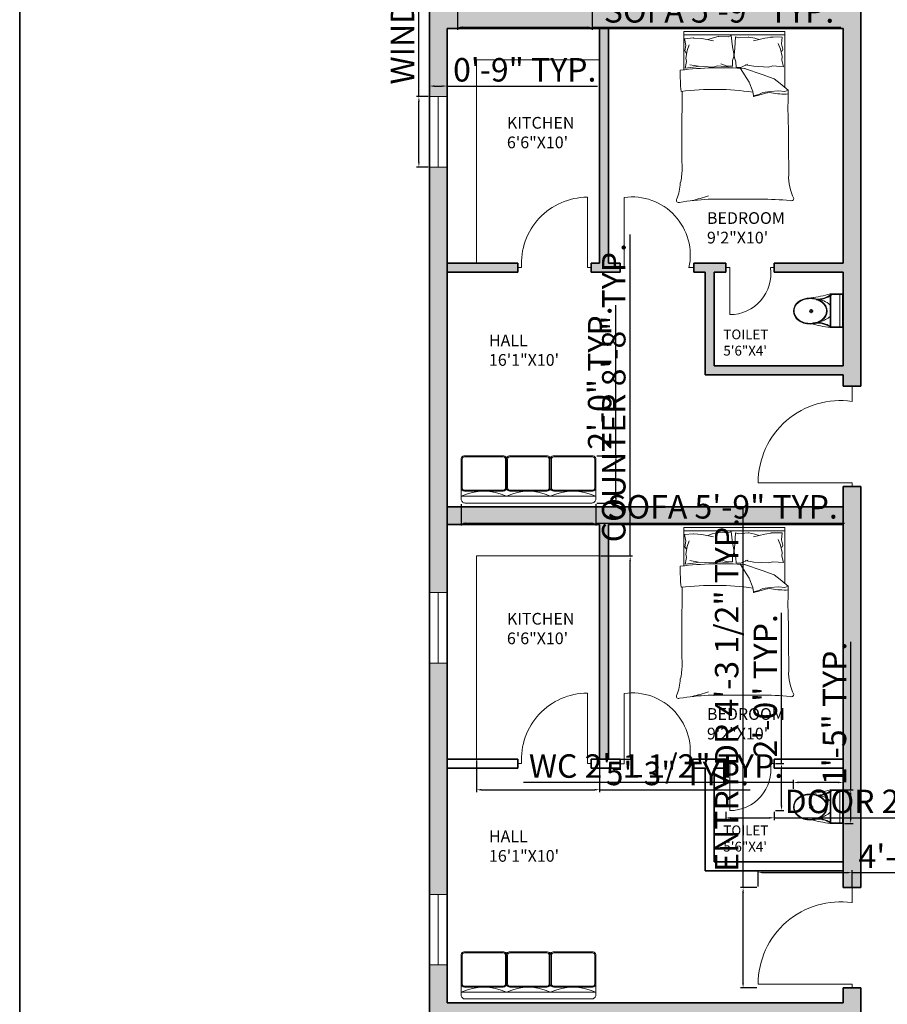
# Model space of a CAD drawing. Units: inches. Extents: x 1266 to 2869, y -408 to 3241.
# Tile 2 of 11: x 1266 to 1710, y 1264 to 1767. Entities that reach past the tile are written whole.
import ezdxf

# ---------------------------------------------------------------- set-up
doc = ezdxf.new("R2010")
doc.units = ezdxf.units.IN
for name, color, linetype, lineweight in [('A-ANNO-DIMS', 2, 'Continuous', 18), ('A-ANNO-TTLB', 7, 'Continuous', 35), ('A-AREA-IDEN', 7, 'Continuous', 18), ('A-DOOR', 4, 'Continuous', 18), ('A-FLOR-CASE', 9, 'Continuous', 18), ('A-FLOR-FIXT', 9, 'Continuous', 18), ('A-FURN', 8, 'Continuous', 18), ('A-GLAZ', 4, 'Continuous', 18), ('A-WALL', 7, 'Continuous', 35), ('A-WALL-PATT', 251, 'Continuous', 13)]:
    doc.layers.add(name, color=color, linetype=linetype, lineweight=lineweight)
doc.styles.get("Standard").update_dxf_attribs({"font": 'arial.ttf'})
doc.dimstyles.new('ISO-25', dxfattribs={"dimtxt": 12, "dimasz": 2.5, "dimexe": 1.25, "dimexo": 0.625, "dimtad": 1, "dimdec": 0, "dimlunit": 3, "dimtxsty": 'Standard', "dimcen": 2.5, "dimadec": 0, "dimazin": 0, "dimtfac": 1, "dimtdec": 0, "dimtmove": 0, "dimatfit": 3, "dimfxl": 1, "dimarcsym": 0})

# ---------------------------------------------------------------- blocks, each defined once
blk = doc.blocks.new('A$C31115884')
for p, q in [((283, 498), (223, 498)), ((258, 466), (258, 523)), ((0, 200), (0, 0)), ((520, 200), (0, 200)), ((10, 190), (10, 10)), ((510, 190), (10, 190)), ((510, 10), (510, 190)), ((520, 0), (520, 200)), ((510, 54), (0, 54)), ((10, 10), (510, 10)), ((0, 0), (520, 0))]:
    blk.add_line(p, q)
blk.add_circle((256, 496), 23.6)
for centre, radius, start, end in [((2778, -205), 2807, 165.4549, 171.7133), ((-295, 403), 365, 324.2091, 9.3499), ((-295, 403), 375, 324.2091, 9.3499), ((806, 403), 365, 170.6501, 215.7909), ((3237, 905), 2807, 188.2867, 194.5451), ((384, 406), 293, 190.2774, 224.1564), ((139, 406), 293, 315.8436, 2.6563), ((806, 403), 375, 179.2036, 215.7909)]:
    blk.add_arc(centre, radius, start, end)
blk.add_ellipse((256, 510), major_axis=(0, -261), ratio=0.772727)
blk.add_open_spline([(256, 259), (263, 259), (270, 260), (288, 262), (299, 265), (320, 273), (330, 278), (350, 291), (360, 299), (378, 316), (386, 326), (402, 347), (409, 358), (421, 383), (427, 395), (436, 422), (440, 436), (445, 465), (447, 480), (448, 509), (448, 524), (445, 553), (443, 568), (436, 596), (432, 610), (422, 636), (416, 649), (402, 672), (395, 683), (379, 703), (370, 712), (351, 728), (341, 735), (321, 746), (310, 751), (289, 757), (278, 759), (256, 761), (245, 761), (223, 757), (212, 754), (191, 746), (181, 741), (161, 728), (151, 720), (133, 703), (125, 693), (110, 672), (103, 660), (90, 636), (85, 623), (76, 596), (72, 582), (67, 553), (66, 538), (64, 509), (65, 494), (68, 465), (70, 450), (77, 422), (81, 408), (91, 382), (97, 370), (111, 346), (118, 335), (135, 316), (144, 307), (162, 291), (172, 284), (193, 273), (203, 269), (225, 262), (236, 260), (250, 259), (253, 259), (256, 259)], degree=3, knots=[0, 0, 0, 0, 0.110105, 0.110105, 0.285049, 0.285049, 0.459994, 0.459994, 0.634938, 0.634938, 0.809882, 0.809882, 0.984827, 0.984827, 1.159771, 1.159771, 1.334715, 1.334715, 1.50966, 1.50966, 1.684604, 1.684604, 1.859549, 1.859549, 2.034493, 2.034493, 2.209437, 2.209437, 2.384382, 2.384382, 2.559326, 2.559326, 2.73427, 2.73427, 2.909215, 2.909215, 3.084159, 3.084159, 3.259103, 3.259103, 3.434048, 3.434048, 3.608992, 3.608992, 3.783936, 3.783936, 3.958881, 3.958881, 4.133825, 4.133825, 4.30877, 4.30877, 4.483714, 4.483714, 4.658658, 4.658658, 4.833603, 4.833603, 5.008547, 5.008547, 5.183491, 5.183491, 5.358436, 5.358436, 5.53338, 5.53338, 5.708324, 5.708324, 5.883269, 5.883269, 6.058213, 6.058213, 6.233158, 6.233158, 6.283185, 6.283185, 6.283185, 6.283185])
blk = doc.blocks.new('BED-DOUBLE')
for p, q in [((3.76, 67.77), (3.76, 87.35)), ((3.76, 87.35), (55.42, 87.35)), ((3.76, 85.69), (55.42, 85.69)), ((55.42, 87.35), (55.42, 58.59)), ((4.21, 83.74), (8.84, 84.1)), ((4.21, 83.77), (4.84, 80.33)), ((5.46, 77.67), (6.55, 80.64)), ((8.84, 84.1), (8.96, 84.08)), ((8.96, 84.08), (13.09, 83.77)), ((13.09, 83.77), (19.03, 82.67)), ((16.06, 83.3), (18.25, 84.08)), ((18.25, 84.08), (21.37, 84.86)), ((21.37, 84.86), (21.72, 84.86)), ((21.72, 84.86), (26.53, 84.7)), ((26.53, 84.7), (28.09, 85.33)), ((28.09, 85.33), (28.71, 79.55)), ((30.24, 84.66), (29.98, 78.85)), ((31.84, 84.13), (30.24, 84.66)), ((36.63, 84.59), (31.84, 84.13)), ((36.98, 84.61), (36.63, 84.59)), ((40.14, 84.02), (36.98, 84.61)), ((45.31, 84.03), (39.45, 82.57)), ((42.38, 83.38), (40.14, 84.02)), ((49.42, 84.6), (45.31, 84.03)), ((54.17, 84.59), (48.33, 84.69)), ((48.33, 84.69), (49.42, 84.6)), ((53.3, 78.43), (52.03, 81.32)), ((54.17, 84.59), (53.76, 81.12)), ((53.76, 81.12), (54.41, 78.34)), ((4.84, 80.33), (4.37, 77.51)), ((4.37, 77.51), (4.99, 76.42)), ((4.84, 73.76), (5.46, 77.67)), ((28.71, 79.55), (29.34, 76.11)), ((29.34, 76.11), (29.34, 74.7)), ((29.98, 78.85), (29.57, 75.38)), ((54.17, 74.56), (53.3, 78.43)), ((54.41, 78.34), (53.85, 77.21)), ((4.52, 68.61), (5.15, 72.04)), ((5.15, 72.04), (4.84, 73.76)), ((26.06, 69.77), (22.66, 70.95)), ((29.34, 74.7), (28.71, 72.67)), ((28.71, 72.67), (28.71, 69.77)), ((29.57, 75.38), (29.66, 73.97)), ((29.66, 73.97), (30.41, 71.98)), ((30.41, 71.98), (30.59, 69.09)), ((33.24, 69.26), (36.56, 70.64)), ((53.97, 72.83), (54.17, 74.56)), ((54.81, 69.44), (53.97, 72.83)), ((10.03, 69.39), (4.52, 68.61)), ((6.9, 70.46), (11.26, 69.74)), ((11.26, 69.74), (10.03, 69.39)), ((11.26, 69.74), (18.84, 69.27)), ((18.84, 69.27), (20.95, 69.87)), ((20.95, 69.87), (26.5, 69.44)), ((28.71, 69.77), (26.06, 69.77)), ((30.59, 69.09), (33.24, 69.26)), ((32.71, 68.56), (37.24, 61.54)), ((43.94, 65.39), (34.92, 68.56)), ((35.2, 70.46), (39.56, 69.74)), ((39.56, 69.74), (47.14, 69.27)), ((47.14, 69.27), (49.26, 69.87)), ((49.26, 69.87), (54.81, 69.44)), ((37.24, 61.54), (39.08, 56.69)), ((49.96, 63.21), (43.94, 65.39)), ((53.15, 60.87), (49.96, 63.21)), ((57.15, 57.36), (53.15, 60.87)), ((39.08, 56.69), (39.42, 54.51)), ((42.1, 55.18), (44.27, 56.19)), ((44.27, 56.19), (47.96, 56.69)), ((47.96, 56.69), (52.14, 57.02)), ((52.14, 57.02), (55.49, 56.69)), ((55.49, 56.69), (57.15, 57.36)), ((57.24, 55.47), (57.15, 57.36, 4.18)), ((39.42, 54.51), (42.1, 55.18)), ((16.28, 1.69), (42.89, 1.69))]:
    blk.add_line(p, q)
for centre, radius, start, end in [((92.06, 65.63), 90.06, 178.7218, 185.604), ((23.09, -109.45), 178.34, 86.0865, 96.7821), ((19.19, -81.63), 139.47, 81.7845, 96.9006), ((-180.86, 53.65), 183.89, 358.4762, 1.0082), ((33.68, 85.75), 32.06, 280.6617, 289.8806), ((47.29, 49.44), 6.73, 78.6608, 113.7384), ((55.49, 94.55), 39.11, 259.8763, 272.5657), ((197.03, 48.09), 139.99, 176.9791, 183.8365), ((39.6, 54.45), 0.199, 160.2464, 271.1377), ((524.11, 32.64), 521.39, 178.2277, 181.7185), ((-4874.07, 14.03), 4931.49, 0.00217, 0.28689), ((-29.08, 17.61), 32.04, 346.0648, 358.9113), ((82.33, 13.12), 24.93, 177.4714, 206.4681), ((-23.41, 11.38), 25.47, 337.9751, 356.652), ((1.18, 1.17), 1.18, 146.1736, 293.4781), ((23.16, -129.76), 131.62, 92.9958, 99.4091), ((-18.62, 112.98), 115.08, 283.3832, 287.7053), ((44.49, -142.13), 143.82, 84.4998, 90.6351), ((58.82, 2.09), 1.19, 242.6588, 356.02)]:
    blk.add_arc(centre, radius, start, end)
blk = doc.blocks.new('SOFA-3-SEAT-3')
for points in [[(0, 22.36), (0, 7.74, 0.414214), (1.72, 6.02), (21.5, 6.02, 0.414214), (23.22, 7.74), (23.22, 22.36, 0.414214), (21.5, 24.08), (1.72, 24.08, 0.414214)], [(0.52, 22.36), (0.52, 7.74, 0.414214), (1.72, 6.54), (21.5, 6.54, 0.414214), (22.7, 7.74), (22.7, 22.36, 0.414214), (21.5, 23.56), (1.72, 23.56, 0.414214)], [(45.57, 22.36), (45.57, 7.74, -0.414214), (43.85, 6.02), (24.94, 6.02, -0.414214), (23.22, 7.74), (23.22, 22.36, -0.414214), (24.94, 24.08), (43.85, 24.08, -0.414214)], [(45.06, 22.36), (45.06, 7.74, -0.414214), (43.85, 6.54), (24.94, 6.54, -0.414214), (23.73, 7.74), (23.73, 22.36, -0.414214), (24.94, 23.56), (43.85, 23.56, -0.414214)], [(45.57, 22.36), (45.57, 7.74, 0.414214), (47.29, 6.02), (67.07, 6.02, 0.414214), (68.79, 7.74), (68.79, 22.36, 0.414214), (67.07, 24.08), (47.29, 24.08, 0.414214)], [(46.09, 22.36), (46.09, 7.74, 0.414214), (47.29, 6.54), (67.07, 6.54, 0.414214), (68.28, 7.74), (68.28, 22.36, 0.414214), (67.07, 23.56), (47.29, 23.56, 0.414214)]]:
    blk.add_lwpolyline(points, format="xyb", close=True)
at = {"ltscale": 0.03}
blk.add_lwpolyline([(21.82, 24.08), (1.38, 24.08, 0.414214), (0, 22.7), (0, 2.06, 0.414214), (2.06, 0), (66.73, 0, 0.414214), (68.79, 2.06), (68.79, 22.7, 0.414214), (67.42, 24.08), (46.97, 24.08, 0.414214), (45.59, 22.7, -1), (45.56, 22.7, 0.414214), (44.18, 24.08), (24.61, 24.08, 0.414214), (23.23, 22.7, -1), (23.2, 22.7, 0.414214)], format="xyb", close=True, dxfattribs=at)
blk.add_lwpolyline([(0, 3.44), (68.79, 3.44)])
for centre, radius, start, end in [((11.61, -21.35), 27.38, 64.9106, 115.0894), ((34.4, -19.35), 25.38, 63.869, 116.131), ((57.18, -21.07), 27.12, 64.6538, 115.3462)]:
    blk.add_arc(centre, radius, start, end)
blk = doc.blocks.new('DOOR-KITCHEN-L')
for p, q in [((35.61, 0), (35.61, 36)), ((0, 0), (2, 0)), ((37.61, 0), (35.61, 0))]:
    blk.add_line(p, q)
blk.add_arc((35.61, 2.31), 33.69, 90, 183.9263)
blk = doc.blocks.new('DOOR-BEDROOM-L')
for p, q in [((2, 0), (2, 36)), ((0, 0), (2, 0)), ((37.12, 0.11), (35.12, 0.11))]:
    blk.add_line(p, q)
blk.add_arc((5.98, 6.45), 29.82, 347.7222, 97.6759)
blk = doc.blocks.new('DOOR-BATH-L')
for p, q in [((0, 24), (2, 24)), ((2, 24), (2, 0)), ((24.7, 24), (22.7, 24))]:
    blk.add_line(p, q)
blk.add_arc((2, 20.92), 20.92, 270, 8.4511)
blk = doc.blocks.new('DOOR-ENTRY-L')
for p, q in [((48, 51.27), (48, 45.59)), ((48, 45.59), (48, 43.59)), ((12, 2), (0, 2)), ((48, 2), (12, 2)), ((48, 0), (48, 2))]:
    blk.add_line(p, q)
blk.add_arc((42.02, 2), 42.02, 81.8116, 180)
blk = doc.blocks.new('WIN-PLAN-36')
for p, q in [((0, 36), (9, 36)), ((4.5, 36), (4.5, 0)), ((9, 36), (4.5, 36)), ((4.5, 0), (0, 0)), ((0, 0), (9, 0))]:
    blk.add_line(p, q)
blk = doc.blocks.new('COUNTER-KITCHEN-2')
for p, q in [((0, 0), (0, 103.95)), ((0, 103.95), (63, 103.95))]:
    blk.add_line(p, q)
blk = doc.blocks.new('*D31')
at = {"layer": 'A-ANNO-DIMS', "color": 0, "lineweight": -2, "transparency": 16777216}
for p, q in [((1470.29, 1727.52), (1470.29, 1883.12)), ((1475.07, 1727.52), (1469.04, 1727.52)), ((1470.29, 1694.02), (1470.29, 1725.02)), ((1475.07, 1691.52), (1469.04, 1691.52))]:
    blk.add_line(p, q, dxfattribs=at)
at = {"layer": 'A-ANNO-DIMS', "color": 0, "transparency": 16777216}
for points in [[(1469.88, 1725.02), (1470.71, 1725.02), (1470.29, 1727.52)], [(1469.88, 1694.02), (1470.71, 1694.02), (1470.29, 1691.52)]]:
    blk.add_solid(points, dxfattribs=at)
at = {"layer": 'Defpoints', "color": 0, "transparency": 16777216}
for p in [(1470.29, 1727.52), (1475.69, 1727.52), (1475.69, 1691.52)]:
    blk.add_point(p, dxfattribs=at)
at = {"layer": 'A-ANNO-DIMS', "color": 0, "transparency": 16777216, "insert": (1463.45, 1806.57), "char_height": 12, "attachment_point": 5, "rotation": 90}
blk.add_mtext('WINDOW 3\'-0" TYP.', dxfattribs=at)
blk = doc.blocks.new('*D32')
at = {"layer": 'A-ANNO-DIMS', "color": 0, "lineweight": -2, "transparency": 16777216}
for p, q in [((1475.69, 1728.15), (1475.69, 1734.17)), ((1478.19, 1732.92), (1482.19, 1732.92)), ((1484.69, 1728.15), (1484.69, 1734.17)), ((1484.69, 1732.92), (1561.59, 1732.92))]:
    blk.add_line(p, q, dxfattribs=at)
at = {"layer": 'A-ANNO-DIMS', "color": 0, "transparency": 16777216}
for points in [[(1478.19, 1733.34), (1478.19, 1732.51), (1475.69, 1732.92)], [(1482.19, 1733.34), (1482.19, 1732.51), (1484.69, 1732.92)]]:
    blk.add_solid(points, dxfattribs=at)
at = {"layer": 'Defpoints', "color": 0, "transparency": 16777216}
for p in [(1484.69, 1732.92), (1475.69, 1727.52), (1484.69, 1727.52)]:
    blk.add_point(p, dxfattribs=at)
at = {"layer": 'A-ANNO-DIMS', "color": 0, "transparency": 16777216, "insert": (1524.39, 1739.68), "char_height": 12, "attachment_point": 5}
blk.add_mtext('0\'-9" TYP.', dxfattribs=at)
blk = doc.blocks.new('*D33')
at = {"layer": 'A-ANNO-DIMS', "color": 0, "lineweight": -2, "transparency": 16777216}
for p, q in [((1661.71, 1376.98), (1523.78, 1376.98)), ((1661.71, 1373.78), (1661.71, 1378.23)), ((1684.69, 1376.98), (1664.21, 1376.98)), ((1687.19, 1373.78), (1687.19, 1378.23))]:
    blk.add_line(p, q, dxfattribs=at)
at = {"layer": 'A-ANNO-DIMS', "color": 0, "transparency": 16777216}
for points in [[(1664.21, 1377.4), (1664.21, 1376.56), (1661.71, 1376.98)], [(1684.69, 1377.4), (1684.69, 1376.56), (1687.19, 1376.98)]]:
    blk.add_solid(points, dxfattribs=at)
at = {"layer": 'Defpoints', "color": 0, "transparency": 16777216}
for p in [(1661.71, 1376.98), (1661.71, 1373.16), (1687.19, 1373.16)]:
    blk.add_point(p, dxfattribs=at)
at = {"layer": 'A-ANNO-DIMS', "color": 0, "transparency": 16777216, "insert": (1591.5, 1383.81), "char_height": 12, "attachment_point": 5}
blk.add_mtext('WC 2\'-1 1/2" TYP.', dxfattribs=at)
blk = doc.blocks.new('*D34')
at = {"layer": 'A-ANNO-DIMS', "color": 0, "lineweight": -2, "transparency": 16777216}
for p, q in [((1691.01, 1373.16), (1691.01, 1448.92)), ((1687.82, 1373.16), (1692.26, 1373.16)), ((1691.01, 1358.46), (1691.01, 1370.66)), ((1687.82, 1355.96), (1692.26, 1355.96))]:
    blk.add_line(p, q, dxfattribs=at)
at = {"layer": 'A-ANNO-DIMS', "color": 0, "transparency": 16777216}
for points in [[(1690.6, 1370.66), (1691.43, 1370.66), (1691.01, 1373.16)], [(1690.6, 1358.46), (1691.43, 1358.46), (1691.01, 1355.96)]]:
    blk.add_solid(points, dxfattribs=at)
at = {"layer": 'Defpoints', "color": 0, "transparency": 16777216}
for p in [(1687.19, 1373.16), (1691.01, 1373.16), (1687.19, 1355.96)]:
    blk.add_point(p, dxfattribs=at)
at = {"layer": 'A-ANNO-DIMS', "color": 0, "transparency": 16777216, "insert": (1684.26, 1412.29), "char_height": 12, "attachment_point": 5, "rotation": 90}
blk.add_mtext('1\'-5" TYP.', dxfattribs=at)
blk = doc.blocks.new('*D35')
at = {"layer": 'A-ANNO-DIMS', "color": 0, "lineweight": -2, "transparency": 16777216}
for p, q in [((1627.24, 1361.97), (1627.24, 1357.64)), ((1629.74, 1358.89), (1649.44, 1358.89)), ((1651.94, 1361.97), (1651.94, 1357.64)), ((1651.94, 1358.89), (1811.15, 1358.89))]:
    blk.add_line(p, q, dxfattribs=at)
at = {"layer": 'A-ANNO-DIMS', "color": 0, "transparency": 16777216}
for points in [[(1629.74, 1359.31), (1629.74, 1358.48), (1627.24, 1358.89)], [(1649.44, 1359.31), (1649.44, 1358.48), (1651.94, 1358.89)]]:
    blk.add_solid(points, dxfattribs=at)
at = {"layer": 'Defpoints', "color": 0, "transparency": 16777216}
for p in [(1627.24, 1362.6), (1651.94, 1362.6), (1651.94, 1358.89)]:
    blk.add_point(p, dxfattribs=at)
at = {"layer": 'A-ANNO-DIMS', "color": 0, "transparency": 16777216, "insert": (1732.8, 1365.73), "char_height": 12, "attachment_point": 5}
blk.add_mtext('DOOR 2\'-0 1/2" TYP.', dxfattribs=at)
blk = doc.blocks.new('*D36')
at = {"layer": 'A-ANNO-DIMS', "color": 0, "lineweight": -2, "transparency": 16777216}
for p, q in [((1655.65, 1386.6), (1655.65, 1463.7)), ((1652.57, 1386.6), (1656.9, 1386.6)), ((1655.65, 1365.1), (1655.65, 1384.1)), ((1652.57, 1362.6), (1656.9, 1362.6))]:
    blk.add_line(p, q, dxfattribs=at)
at = {"layer": 'A-ANNO-DIMS', "color": 0, "transparency": 16777216}
for points in [[(1655.23, 1384.1), (1656.06, 1384.1), (1655.65, 1386.6)], [(1655.23, 1365.1), (1656.06, 1365.1), (1655.65, 1362.6)]]:
    blk.add_solid(points, dxfattribs=at)
at = {"layer": 'Defpoints', "color": 0, "transparency": 16777216}
for p in [(1651.94, 1386.6), (1655.65, 1386.6), (1651.94, 1362.6)]:
    blk.add_point(p, dxfattribs=at)
at = {"layer": 'A-ANNO-DIMS', "color": 0, "transparency": 16777216, "insert": (1648.89, 1426.4), "char_height": 12, "attachment_point": 5, "rotation": 90}
blk.add_mtext('2\'-0" TYP.', dxfattribs=at)
blk = doc.blocks.new('*D45')
at = {"layer": 'A-ANNO-DIMS', "color": 0, "lineweight": -2, "transparency": 16777216}
for p, q in [((1636, 1323.21), (1636, 1517.78)), ((1643.07, 1323.21), (1634.75, 1323.21)), ((1636, 1274.44), (1636, 1320.71)), ((1643.07, 1271.94), (1634.75, 1271.94))]:
    blk.add_line(p, q, dxfattribs=at)
at = {"layer": 'A-ANNO-DIMS', "color": 0, "transparency": 16777216}
for points in [[(1635.58, 1320.71), (1636.42, 1320.71), (1636, 1323.21)], [(1635.58, 1274.44), (1636.42, 1274.44), (1636, 1271.94)]]:
    blk.add_solid(points, dxfattribs=at)
at = {"layer": 'Defpoints', "color": 0, "transparency": 16777216}
for p in [(1636, 1323.21), (1643.69, 1323.21), (1643.69, 1271.94)]:
    blk.add_point(p, dxfattribs=at)
at = {"layer": 'A-ANNO-DIMS', "color": 0, "transparency": 16777216, "insert": (1629.17, 1421.75), "char_height": 12, "attachment_point": 5, "rotation": 90}
blk.add_mtext('ENTRY DR 4\'-3 1/2" TYP.', dxfattribs=at)
blk = doc.blocks.new('*D46')
at = {"layer": 'A-ANNO-DIMS', "color": 0, "lineweight": -2, "transparency": 16777216}
for p, q in [((1643.69, 1323.83), (1643.69, 1332.15)), ((1646.19, 1330.9), (1689.19, 1330.9)), ((1691.69, 1323.83), (1691.69, 1332.15)), ((1691.69, 1330.9), (1769.07, 1330.9))]:
    blk.add_line(p, q, dxfattribs=at)
at = {"layer": 'A-ANNO-DIMS', "color": 0, "transparency": 16777216}
for points in [[(1646.19, 1331.32), (1646.19, 1330.48), (1643.69, 1330.9)], [(1689.19, 1331.32), (1689.19, 1330.48), (1691.69, 1330.9)]]:
    blk.add_solid(points, dxfattribs=at)
at = {"layer": 'Defpoints', "color": 0, "transparency": 16777216}
for p in [(1691.69, 1330.9), (1643.69, 1323.21), (1691.69, 1323.21)]:
    blk.add_point(p, dxfattribs=at)
at = {"layer": 'A-ANNO-DIMS', "color": 0, "transparency": 16777216, "insert": (1731.63, 1337.65), "char_height": 12, "attachment_point": 5}
blk.add_mtext('4\'-0" TYP.', dxfattribs=at)
blk = doc.blocks.new('*D63')
at = {"layer": 'A-ANNO-DIMS', "color": 0, "lineweight": -2, "transparency": 16777216}
for p, q in [((1578.28, 1492.79), (1578.28, 1657.1)), ((1563.32, 1492.79), (1579.53, 1492.79)), ((1578.28, 1391.35), (1578.28, 1490.29)), ((1563.32, 1388.85), (1579.53, 1388.85))]:
    blk.add_line(p, q, dxfattribs=at)
at = {"layer": 'A-ANNO-DIMS', "color": 0, "transparency": 16777216}
for points in [[(1577.87, 1490.29), (1578.7, 1490.29), (1578.28, 1492.79)], [(1577.87, 1391.35), (1578.7, 1391.35), (1578.28, 1388.85)]]:
    blk.add_solid(points, dxfattribs=at)
at = {"layer": 'Defpoints', "color": 0, "transparency": 16777216}
for p in [(1562.69, 1492.79), (1578.28, 1492.79), (1562.69, 1388.85)]:
    blk.add_point(p, dxfattribs=at)
at = {"layer": 'A-ANNO-DIMS', "color": 0, "transparency": 16777216, "insert": (1571.45, 1576.2), "char_height": 12, "attachment_point": 5, "rotation": 90}
blk.add_mtext('COUNTER 8\'-8" TYP.', dxfattribs=at)
blk = doc.blocks.new('*D64')
at = {"layer": 'A-ANNO-DIMS', "color": 0, "lineweight": -2, "transparency": 16777216}
for p, q in [((1499.69, 1388.22), (1499.69, 1372)), ((1562.69, 1388.22), (1562.69, 1372)), ((1502.19, 1373.25), (1560.19, 1373.25)), ((1562.69, 1373.25), (1639.59, 1373.25))]:
    blk.add_line(p, q, dxfattribs=at)
at = {"layer": 'A-ANNO-DIMS', "color": 0, "transparency": 16777216}
for points in [[(1502.19, 1373.67), (1502.19, 1372.84), (1499.69, 1373.25)], [(1560.19, 1373.67), (1560.19, 1372.84), (1562.69, 1373.25)]]:
    blk.add_solid(points, dxfattribs=at)
at = {"layer": 'Defpoints', "color": 0, "transparency": 16777216}
for p in [(1499.69, 1388.85), (1562.69, 1388.85), (1562.69, 1373.25)]:
    blk.add_point(p, dxfattribs=at)
at = {"layer": 'A-ANNO-DIMS', "color": 0, "transparency": 16777216, "insert": (1602.39, 1380.01), "char_height": 12, "attachment_point": 5}
blk.add_mtext('5\'-3" TYP.', dxfattribs=at)
blk = doc.blocks.new('*D67')
at = {"layer": 'A-ANNO-DIMS', "color": 0, "lineweight": -2, "transparency": 16777216}
for p, q in [((1490.09, 1772.67), (1490.09, 1761.73)), ((1558.88, 1772.67), (1558.88, 1761.73)), ((1492.59, 1762.98), (1556.38, 1762.98)), ((1558.88, 1762.98), (1686.02, 1762.98))]:
    blk.add_line(p, q, dxfattribs=at)
at = {"layer": 'A-ANNO-DIMS', "color": 0, "transparency": 16777216}
for points in [[(1492.59, 1763.4), (1492.59, 1762.56), (1490.09, 1762.98)], [(1556.38, 1763.4), (1556.38, 1762.56), (1558.88, 1762.98)]]:
    blk.add_solid(points, dxfattribs=at)
at = {"layer": 'Defpoints', "color": 0, "transparency": 16777216}
for p in [(1490.09, 1773.3), (1558.88, 1773.3), (1558.88, 1762.98)]:
    blk.add_point(p, dxfattribs=at)
at = {"layer": 'A-ANNO-DIMS', "color": 0, "transparency": 16777216, "insert": (1623.7, 1769.81), "char_height": 12, "attachment_point": 5}
blk.add_mtext('SOFA 5\'-9" TYP.', dxfattribs=at)
blk = doc.blocks.new('*D71')
at = {"layer": 'A-ANNO-DIMS', "color": 0, "lineweight": -2, "transparency": 16777216}
for p, q in [((1491.9, 1519.17), (1491.9, 1508.23)), ((1560.69, 1519.17), (1560.69, 1508.23)), ((1494.4, 1509.48), (1558.19, 1509.48)), ((1560.69, 1509.48), (1687.83, 1509.48))]:
    blk.add_line(p, q, dxfattribs=at)
at = {"layer": 'A-ANNO-DIMS', "color": 0, "transparency": 16777216}
for points in [[(1494.4, 1509.9), (1494.4, 1509.06), (1491.9, 1509.48)], [(1558.19, 1509.9), (1558.19, 1509.06), (1560.69, 1509.48)]]:
    blk.add_solid(points, dxfattribs=at)
at = {"layer": 'Defpoints', "color": 0, "transparency": 16777216}
for p in [(1491.9, 1519.8), (1560.69, 1519.8), (1560.69, 1509.48)]:
    blk.add_point(p, dxfattribs=at)
at = {"layer": 'A-ANNO-DIMS', "color": 0, "transparency": 16777216, "insert": (1625.51, 1516.31), "char_height": 12, "attachment_point": 5}
blk.add_mtext('SOFA 5\'-9" TYP.', dxfattribs=at)
blk = doc.blocks.new('*D72')
at = {"layer": 'A-ANNO-DIMS', "color": 0, "lineweight": -2, "transparency": 16777216}
for p, q in [((1571.01, 1543.88), (1571.01, 1620.98)), ((1561.32, 1543.88), (1572.26, 1543.88)), ((1571.01, 1522.3), (1571.01, 1541.38)), ((1561.32, 1519.8), (1572.26, 1519.8))]:
    blk.add_line(p, q, dxfattribs=at)
at = {"layer": 'A-ANNO-DIMS', "color": 0, "transparency": 16777216}
for points in [[(1570.59, 1541.38), (1571.43, 1541.38), (1571.01, 1543.88)], [(1570.59, 1522.3), (1571.43, 1522.3), (1571.01, 1519.8)]]:
    blk.add_solid(points, dxfattribs=at)
at = {"layer": 'Defpoints', "color": 0, "transparency": 16777216}
for p in [(1560.69, 1543.88), (1571.01, 1543.88), (1560.69, 1519.8)]:
    blk.add_point(p, dxfattribs=at)
at = {"layer": 'A-ANNO-DIMS', "color": 0, "transparency": 16777216, "insert": (1564.26, 1583.68), "char_height": 12, "attachment_point": 5, "rotation": 90}
blk.add_mtext('2\'-0" TYP.', dxfattribs=at)

msp = doc.modelspace()

# ---------------------------------------------------------------- hatches: boundary and pattern name
at = {"layer": 'A-WALL-PATT'}
h = msp.add_hatch(color=256, dxfattribs=at)
h.dxf.hatch_style = 1
h.paths.add_polyline_path([(1484.69, 2269.35), (1562.69, 2269.35), (1562.69, 2149.35), (1558.42, 2149.35), (1558.42, 2144.85), (1567.19, 2144.85), (1573.23, 2144.85), (1573.23, 2146.74), (1573.23, 2149.35), (1567.19, 2149.35), (1567.19, 2269.35), (1597.45, 2269.35), (1597.45, 2273.85), (1597.45, 2278.35), (1475.69, 2278.35), (1475.69, 2234.52), (1484.69, 2234.52)])
h.paths.add_polyline_path([(1873.25, 2278.35), (1748.19, 2278.35), (1696.19, 2278.35), (1657.45, 2278.35), (1657.45, 2269.35), (1687.19, 2269.35), (1687.19, 2149.35), (1651.94, 2149.35), (1651.94, 2144.85), (1687.19, 2144.85), (1687.19, 2133.61), (1696.19, 2133.61), (1696.19, 2269.35), (1748.19, 2269.35), (1748.19, 2234.52), (1757.19, 2234.52), (1757.19, 2269.35), (1835.19, 2269.35), (1835.19, 2149.35), (1827.33, 2149.35), (1827.33, 2144.85), (1843.74, 2144.85), (1843.74, 2149.35), (1839.69, 2149.35), (1839.69, 2269.35), (1873.25, 2269.35), (1873.25, 2273.85)])
h.paths.add_polyline_path([(1958.69, 2278.35), (1933.25, 2278.35), (1933.25, 2269.35), (1949.69, 2269.35), (1949.69, 2149.35), (1912.22, 2149.35), (1912.22, 2144.85), (1949.69, 2144.85), (1949.69, 2133.61), (1958.69, 2133.61)])
h.paths.add_polyline_path([(1883.69, 2144.85), (1889.08, 2144.85), (1889.08, 2149.35), (1875.58, 2149.35), (1875.58, 2144.85), (1879.19, 2144.85), (1879.19, 2092.35), (1949.69, 2092.35), (1949.69, 2086.89), (1949.69, 2024.85), (1933.25, 2024.85), (1933.25, 2015.85), (1949.69, 2015.85), (1949.69, 1895.85), (1912.45, 1895.85), (1912.45, 1891.35), (1949.69, 1891.35), (1949.69, 1880.11), (1958.69, 1880.11), (1958.69, 2086.89), (1958.69, 2109.61), (1949.69, 2109.61), (1949.69, 2096.85), (1883.69, 2096.85)])
h.paths.add_polyline_path([(1757.19, 2198.52), (1748.19, 2198.52), (1748.19, 2086.89), (1757.19, 2086.89), (1757.19, 2144.85), (1793.55, 2144.85), (1793.55, 2149.35), (1757.19, 2149.35)])
h.paths.add_polyline_path([(1696.19, 2109.61), (1687.19, 2109.61), (1687.19, 2096.85), (1621.19, 2096.85), (1621.19, 2144.85), (1627.24, 2144.85), (1627.24, 2149.35), (1616.69, 2149.35), (1610.35, 2149.35), (1610.35, 2144.85), (1616.69, 2144.85), (1616.69, 2092.35), (1687.19, 2092.35), (1687.19, 2086.89), (1696.19, 2086.89)], flags=17)
h.paths.add_polyline_path([(1484.69, 2144.85), (1520.8, 2144.85), (1520.8, 2149.35), (1484.69, 2149.35), (1484.69, 2198.52), (1475.69, 2198.52), (1475.69, 1981.02), (1484.69, 1981.02), (1484.69, 2015.85), (1687.19, 2015.85), (1687.19, 1895.85), (1650.13, 1895.85), (1650.13, 1891.35), (1687.19, 1891.35), (1687.19, 1880.11), (1696.19, 1880.11), (1696.19, 2035.62), (1687.19, 2035.62), (1687.19, 2024.85), (1484.69, 2024.85)])
h.paths.add_polyline_path([(1484.69, 1691.52), (1475.69, 1691.52), (1475.69, 1474.02), (1484.69, 1474.02)])
h.paths.add_polyline_path([(1518.03, 1895.85), (1484.69, 1895.85), (1484.69, 1945.02), (1475.69, 1945.02), (1475.69, 1727.52), (1484.69, 1727.52), (1484.69, 1762.35), (1687.19, 1762.35), (1687.19, 1642.35), (1651.94, 1642.35), (1651.94, 1637.85), (1687.19, 1637.85), (1687.19, 1589.85), (1621.19, 1589.85), (1621.19, 1637.85), (1627.19, 1637.85), (1627.19, 1642.35), (1610.89, 1642.35), (1610.89, 1637.85), (1616.69, 1637.85), (1616.69, 1585.35), (1687.19, 1585.35), (1687.19, 1579.45), (1696.19, 1579.45), (1696.19, 1779.84), (1687.19, 1779.84), (1687.19, 1771.35), (1484.69, 1771.35), (1484.69, 1891.35), (1518.03, 1891.35)])
h.paths.add_polyline_path([(1567.19, 2015.85), (1562.69, 2015.85), (1562.69, 1895.85), (1555.64, 1895.85), (1555.64, 1891.35), (1570.46, 1891.35), (1570.46, 1895.85), (1567.19, 1895.85)], flags=17)
h.paths.add_polyline_path([(1625.43, 1895.85), (1607.58, 1895.85), (1607.58, 1891.35), (1616.69, 1891.35), (1616.69, 1838.85), (1687.19, 1838.85), (1687.19, 1831.11), (1696.19, 1831.11), (1696.19, 1856.11), (1687.19, 1856.11), (1687.19, 1843.35), (1621.19, 1843.35), (1621.19, 1891.35), (1625.43, 1891.35)], flags=17)
h.paths.add_polyline_path([(1567.19, 1762.35), (1562.69, 1762.35), (1562.69, 1642.35), (1558.42, 1642.35), (1558.42, 1637.85), (1573.23, 1637.85), (1573.23, 1642.35), (1567.19, 1642.35)], flags=17)
h.paths.add_polyline_path([(1520.8, 1642.35), (1484.69, 1642.35), (1484.69, 1637.85), (1520.8, 1637.85)], flags=17)
h.paths.add_polyline_path([(1687.19, 1517.85), (1484.69, 1517.85), (1484.69, 1508.85), (1562.69, 1508.85), (1562.69, 1388.85), (1567.19, 1388.85), (1567.19, 1508.85), (1687.19, 1508.85)])
h.paths.add_polyline_path([(1696.19, 1528.18), (1687.19, 1528.18), (1687.19, 1323.21), (1696.19, 1323.21)])
h.paths.add_polyline_path([(1696.19, 1271.94), (1687.19, 1271.94), (1687.19, 1264.35), (1484.69, 1264.35), (1484.69, 1283.77), (1480.19, 1283.77), (1475.69, 1283.77), (1475.69, 1255.35), (1480.19, 1255.35), (1696.19, 1255.35)])
h.paths.add_polyline_path([(1484.69, 1438.02), (1475.69, 1438.02), (1475.69, 1319.77), (1484.69, 1319.77)])
h.paths.add_polyline_path([(1873.25, 1513.35), (1873.25, 1517.85), (1757.19, 1517.85), (1757.19, 1528.62), (1748.19, 1528.62), (1748.19, 1474.02), (1757.19, 1474.02), (1757.19, 1508.85), (1835.19, 1508.85), (1835.19, 1388.85), (1827.33, 1388.85), (1827.33, 1384.35), (1843.74, 1384.35), (1843.74, 1388.85), (1839.69, 1388.85), (1839.69, 1508.85), (1873.25, 1508.85)])
h.paths.add_polyline_path([(1958.69, 1602.61), (1949.69, 1602.61), (1949.69, 1517.85), (1933.25, 1517.85), (1933.25, 1508.85), (1949.69, 1508.85), (1949.69, 1388.85), (1912.22, 1388.85), (1912.22, 1384.35), (1949.69, 1384.35), (1949.69, 1373.11), (1958.69, 1373.11)])
h.paths.add_polyline_path([(1958.69, 1349.11), (1949.69, 1349.11), (1949.69, 1336.35), (1883.69, 1336.35), (1883.69, 1384.35), (1889.08, 1384.35), (1889.08, 1388.85), (1875.58, 1388.85), (1875.58, 1384.35), (1879.19, 1384.35), (1879.19, 1331.85), (1949.69, 1331.85), (1949.69, 1315.59), (1958.69, 1315.59)])
h.paths.add_polyline_path([(1958.69, 1279.59), (1954.19, 1279.59), (1949.69, 1279.59), (1949.69, 1264.35), (1757.19, 1264.35), (1757.19, 1275.12), (1748.19, 1275.12), (1748.19, 1255.35), (1958.69, 1255.35)])
h.paths.add_polyline_path([(1757.19, 1438.02), (1748.19, 1438.02), (1748.19, 1326.39), (1757.19, 1326.39)])
h.paths.add_polyline_path([(1793.55, 1388.85), (1757.19, 1388.85), (1757.19, 1384.35), (1793.55, 1384.35)], flags=0)

# ---------------------------------------------------------------- linework, layer by layer
at = {"layer": 'A-ANNO-TTLB'}
msp.add_lwpolyline([(1266.23, 3241.34), (2868.62, 3241.34), (2868.62, 986.84), (1266.23, 986.84)], close=True, dxfattribs=at)
at = {"layer": 'A-DOOR'}
for p, q in [((1575.23, 1639.99), (1575.23, 1675.99)), ((1573.23, 1639.99), (1575.23, 1639.99)), ((1608.35, 1640.1), (1608.89, 1640.1)), ((1608.89, 1640.1), (1610.89, 1640.1))]:
    msp.add_line(p, q, dxfattribs=at)
msp.add_arc((1579.21, 1646.44), 29.82, 347.7222, 97.6759, dxfattribs=at)
at = {"layer": 'A-WALL'}
for p, q in [((1475.69, 2278.35), (1475.69, 1255.35)), ((1696.19, 1779.84), (1696.19, 1579.45)), ((1484.69, 1762.35), (1687.19, 1762.35)), ((1484.69, 1762.35), (1484.69, 1264.35)), ((1562.69, 1762.35), (1562.69, 1642.35)), ((1562.69, 1762.35), (1562.69, 1642.35)), ((1567.19, 1762.35), (1567.19, 1642.35)), ((1567.19, 1762.35), (1567.19, 1642.35)), ((1687.19, 1762.35), (1687.19, 1642.35)), ((1484.69, 1642.35), (1520.8, 1642.35)), ((1520.8, 1640.1), (1520.8, 1642.35)), ((1520.8, 1642.35), (1520.8, 1637.85)), ((1558.42, 1640.1), (1558.42, 1642.35)), ((1558.42, 1642.35), (1558.42, 1637.85)), ((1558.42, 1642.35), (1562.69, 1642.35)), ((1567.19, 1642.35), (1573.23, 1642.35)), ((1573.23, 1639.99), (1573.23, 1642.35)), ((1573.23, 1642.35), (1573.23, 1637.85)), ((1610.89, 1640.1), (1610.89, 1642.35)), ((1610.89, 1642.35), (1610.89, 1637.85)), ((1610.89, 1642.35), (1627.19, 1642.35)), ((1627.24, 1640.1), (1627.19, 1642.35)), ((1627.19, 1642.35), (1627.19, 1637.85)), ((1651.94, 1640.1), (1651.94, 1642.35)), ((1651.94, 1642.35), (1651.94, 1637.85)), ((1651.94, 1642.35), (1687.19, 1642.35)), ((1484.69, 1637.85), (1520.8, 1637.85)), ((1558.42, 1637.85), (1573.23, 1637.85)), ((1610.89, 1637.85), (1616.69, 1637.85)), ((1616.69, 1637.85), (1616.69, 1585.35)), ((1621.19, 1637.85), (1621.19, 1589.85)), ((1621.19, 1637.85), (1627.19, 1637.85)), ((1651.94, 1637.85), (1687.19, 1637.85)), ((1687.19, 1637.85), (1687.19, 1589.85)), ((1616.69, 1585.35), (1687.19, 1585.35)), ((1621.19, 1589.85), (1687.19, 1589.85)), ((1687.19, 1585.35), (1687.19, 1579.45)), ((1691.69, 1579.45), (1687.19, 1579.45)), ((1687.19, 1579.45), (1696.19, 1579.45)), ((1691.69, 1528.18), (1687.19, 1528.18)), ((1687.19, 1528.18), (1696.19, 1528.18)), ((1687.19, 1528.18), (1687.19, 1323.21)), ((1696.19, 1528.18), (1696.19, 1323.21)), ((1484.69, 1517.85), (1687.19, 1517.85)), ((1484.69, 1508.85), (1562.69, 1508.85)), ((1562.69, 1508.85), (1562.69, 1388.85)), ((1567.19, 1508.85), (1567.19, 1388.85)), ((1567.19, 1508.85), (1687.19, 1508.85)), ((1484.69, 1388.85), (1520.8, 1388.85)), ((1484.69, 1384.35), (1520.8, 1384.35)), ((1520.8, 1386.6), (1520.8, 1388.85)), ((1520.8, 1388.85), (1520.8, 1384.35)), ((1558.42, 1386.6), (1558.42, 1388.85)), ((1558.42, 1388.85), (1558.42, 1384.35)), ((1558.42, 1388.85), (1573.23, 1388.85)), ((1558.42, 1384.35), (1573.23, 1384.35)), ((1573.23, 1386.49), (1573.23, 1388.85)), ((1573.23, 1388.85), (1573.23, 1384.35)), ((1610.35, 1386.6), (1610.35, 1388.85)), ((1610.35, 1388.85), (1610.35, 1384.35)), ((1610.35, 1388.85), (1627.24, 1388.85)), ((1610.35, 1384.35), (1616.69, 1384.35)), ((1616.69, 1384.35), (1616.69, 1331.85)), ((1621.19, 1384.35), (1621.19, 1336.35)), ((1621.19, 1384.35), (1627.24, 1384.35)), ((1627.24, 1386.6), (1627.24, 1388.85)), ((1627.24, 1388.85), (1627.24, 1384.35)), ((1627.24, 1384.35), (1627.24, 1384.35)), ((1651.94, 1386.6), (1651.94, 1388.85)), ((1651.94, 1388.85), (1651.94, 1384.35)), ((1651.94, 1388.85), (1687.19, 1388.85)), ((1651.94, 1384.35), (1687.19, 1384.35)), ((1621.19, 1336.35), (1687.19, 1336.35)), ((1616.69, 1331.85), (1687.19, 1331.85)), ((1691.69, 1323.21), (1687.19, 1323.21)), ((1687.19, 1323.21), (1696.19, 1323.21)), ((1691.69, 1271.94), (1687.19, 1271.94)), ((1687.19, 1271.94), (1696.19, 1271.94)), ((1687.19, 1271.94), (1687.19, 1264.35)), ((1696.19, 1271.94), (1696.19, 1255.35)), ((1484.69, 1264.35), (1687.19, 1264.35))]:
    msp.add_line(p, q, dxfattribs=at)

# ---------------------------------------------------------------- block references
at = {"layer": 'A-DOOR'}
for name, p in [('DOOR-KITCHEN-L', (1520.8, 1640.1)), ('DOOR-BATH-L', (1627.24, 1616.1)), ('DOOR-ENTRY-L', (1643.69, 1528.18)), ('DOOR-KITCHEN-L', (1520.8, 1386.6)), ('DOOR-BEDROOM-L', (1573.23, 1386.49)), ('DOOR-BATH-L', (1627.24, 1362.6)), ('DOOR-ENTRY-L', (1643.69, 1271.94))]:
    msp.add_blockref(name, p, dxfattribs=at)
at = {"layer": 'A-FLOR-CASE'}
for p in [(1499.69, 1642.35), (1499.69, 1388.85)]:
    msp.add_blockref('COUNTER-KITCHEN-2', p, dxfattribs=at)
at = {"layer": 'A-FLOR-FIXT', "xscale": 0.0330640103915726, "yscale": 0.0330640103915726, "zscale": 0.0330640103915726, "rotation": 89.99999999999996}
for p in [(1687.19, 1609.46), (1687.19, 1355.96)]:
    msp.add_blockref('A$C31115884', p, dxfattribs=at)
at = {"layer": 'A-FURN'}
for name, p in [('BED-DOUBLE', (1601.89, 1673.39)), ('SOFA-3-SEAT-3', (1491.9, 1519.8)), ('BED-DOUBLE', (1601.89, 1419.89)), ('SOFA-3-SEAT-3', (1491.9, 1266.3))]:
    msp.add_blockref(name, p, dxfattribs=at)
at = {"layer": 'A-GLAZ'}
for p in [(1475.69, 1691.52), (1475.69, 1438.02)]:
    msp.add_blockref('WIN-PLAN-36', p, dxfattribs=at)
at = {"layer": 'A-GLAZ', "rotation": 180}
msp.add_blockref('WIN-PLAN-36', (1484.69, 1319.77), dxfattribs=at)

# ---------------------------------------------------------------- texts
at = {"layer": 'A-AREA-IDEN', "attachment_point": 1}
for s, width, insert, char_height in [('KITCHEN\\P6\'6"X10\'', 112.1355, (1515.28, 1717.14), 6), ('BEDROOM\\P9\'2"X10\'', 62.026, (1617.54, 1668.46), 6), ('HALL\\P16\'1"X10\'', 100.9767, (1506.1, 1605.93), 6), ('TOILET\\P5\'6"X4\'', 46.3569, (1625.93, 1608.49), 5), ('KITCHEN\\P6\'6"X10\'', 112.1355, (1515.28, 1463.64), 6), ('BEDROOM\\P9\'2"X10\'', 62.026, (1617.54, 1414.96), 6), ('TOILET\\P5\'6"X4\'', 46.3569, (1625.93, 1354.99), 5), ('HALL\\P16\'1"X10\'', 100.9767, (1506.1, 1352.43), 6)]:
    msp.add_mtext_dynamic_manual_height_columns(s, width=width, gutter_width=12.5, heights=[0], dxfattribs=dict(at, insert=insert, char_height=char_height))

# ---------------------------------------------------------------- dimensions: what is measured, and where the dimension line sits
at = {"layer": 'A-ANNO-DIMS'}
for base, p1, p2, angle, text, picture, middle in [((1470.29, 1727.52), (1475.69, 1691.52), (1475.69, 1727.52), 90, 'WINDOW <> TYP.', '*D31', (1463.45, 1806.57)), ((1578.28, 1492.79), (1562.69, 1388.85), (1562.69, 1492.79), 90, 'COUNTER <> TYP.', '*D63', (1571.45, 1576.2)), ((1571.01, 1543.88), (1560.69, 1519.8), (1560.69, 1543.88), 90, '<> TYP.', '*D72', (1564.26, 1583.68)), ((1636, 1323.21), (1643.69, 1271.94), (1643.69, 1323.21), 90, 'ENTRY DR <> TYP.', '*D45', (1629.17, 1421.75)), ((1655.65, 1386.6), (1651.94, 1362.6), (1651.94, 1386.6), 90, '<> TYP.', '*D36', (1648.89, 1426.4)), ((1691.01, 1373.16), (1687.19, 1355.96), (1687.19, 1373.16), 90, '<> TYP.', '*D34', (1684.26, 1412.29)), ((1661.71, 1376.98), (1687.19, 1373.16), (1661.71, 1373.16), 180, 'WC <> TYP.', '*D33', (1591.5, 1383.81))]:
    dim = msp.add_linear_dim(base=base, p1=p1, p2=p2, angle=angle, text=text, dimstyle='ISO-25', override={"dimdec": 1, "dimlfac": 1, "dimrnd": 0, "dimzin": 1, "dimdsep": 46, "dimlunit": 4, "dimfrac": 2}, dxfattribs=at)
    dim.commit()
    dim.dimension.update_dxf_attribs({"geometry": picture, "text_midpoint": middle})
for base, p1, p2, text, picture, middle in [((1558.88, 1762.98), (1490.09, 1773.3), (1558.88, 1773.3), 'SOFA <> TYP.', '*D67', (1623.7, 1769.81)), ((1484.69, 1732.92), (1475.69, 1727.52), (1484.69, 1727.52), '<> TYP.', '*D32', (1524.39, 1739.68)), ((1560.69, 1509.48), (1491.9, 1519.8), (1560.69, 1519.8), 'SOFA <> TYP.', '*D71', (1625.51, 1516.31)), ((1651.94, 1358.89), (1627.24, 1362.6), (1651.94, 1362.6), 'DOOR <> TYP.', '*D35', (1732.8, 1365.73)), ((1562.69, 1373.25), (1499.69, 1388.85), (1562.69, 1388.85), '<> TYP.', '*D64', (1602.39, 1380.01)), ((1691.69, 1330.9), (1643.69, 1323.21), (1691.69, 1323.21), '<> TYP.', '*D46', (1731.63, 1337.65))]:
    dim = msp.add_linear_dim(base=base, p1=p1, p2=p2, text=text, dimstyle='ISO-25', override={"dimdec": 1, "dimlfac": 1, "dimrnd": 0, "dimzin": 1, "dimdsep": 46, "dimlunit": 4, "dimfrac": 2}, dxfattribs=at)
    dim.commit()
    dim.dimension.update_dxf_attribs({"geometry": picture, "text_midpoint": middle})

doc.saveas('drawing.dxf')
